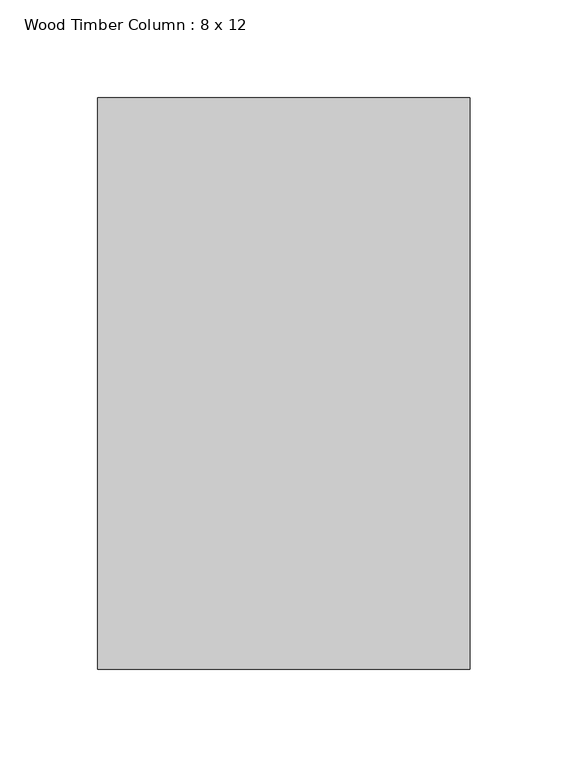
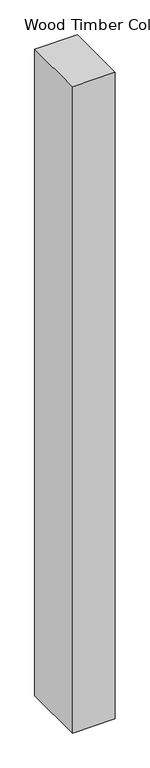
"""IFC4 building model written with IfcOpenShell, lengths in millimetres: column geometry, Wood Timber Column : 8 x 12."""

from ifc_helpers import new_model, si_unit, origin, origin_with_axes, place, context, project, spatial, polyline, outline, extrude, source, transform, mapped, element, save


def wood_timber_column_8_x_12_245a0583(model_context):
    return source(origin(), model_context, "Body", "SweptSolid", [
        extrude(outline(polyline([(95.25, -146.05), (-95.25, -146.05), (-95.25, 146.05), (95.25, 146.05), (95.25, -146.05)])), origin_with_axes(), (0.0, 0.0, 1.0), 3048.0),
    ])


if __name__ == "__main__":
    model = new_model("IFC4")
    model_context = context("Model", 3, world=origin())
    ifc_project = project(units=[si_unit("LENGTHUNIT", "METRE", prefix="MILLI")], contexts=[model_context])
    site = spatial("IfcSite", under=ifc_project)
    building = spatial("IfcBuilding", under=site)
    placement = place(None, origin())
    wood_timber_column_8_x_12_shape = wood_timber_column_8_x_12_245a0583(model_context)
    element("IfcColumn", 1, ObjectType="Wood Timber Column : 8 x 12", at=placement, inside=building, context=model_context, shape_type="MappedRepresentation", body=[
        mapped(wood_timber_column_8_x_12_shape, transform((0.0, 0.0, 0.0), x_axis=(1.0, 0.0, 0.0), y_axis=(0.0, 1.0, 0.0), z_axis=(0.0, 0.0, 1.0))),
    ])
    save(model, "model.ifc")

# Revit data of these elements
# Type "Wood Timber Column : 8 x 12"
#   Assembly Code = "B1010200"
#   Depth = 0' - 11 1/2"
#   Width = 0' - 7 1/2"
#   Material = Rigid insulation
# Element 1 (IfcColumn, "Wood Timber Column : 8 x 12")
#   Materials on its faces: "Rigid insulation"
# Materials
#   "Rigid insulation": class "Generic", colour RGB 127 127 127, transparency 0, Description = "Rigid foam insulation board", Cost = 0
